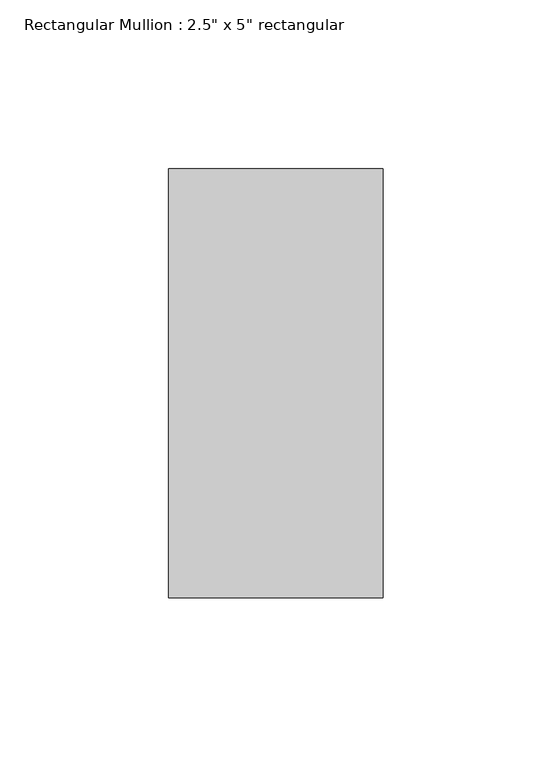
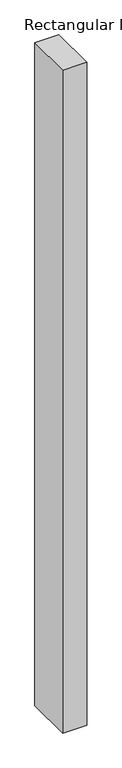
"""IFC4 building model written with IfcOpenShell, lengths in millimetres: member geometry."""

from ifc_helpers import new_model, si_unit, frame, origin, place, context, project, spatial, polyline, outline, extrude, source, transform, mapped, element, save


def member_d73967ec(model_context):
    return source(origin(), model_context, "Body", "SweptSolid", [
        extrude(outline(polyline([(31.75, 63.5), (31.75, -63.5), (-31.75, -63.5), (-31.75, 63.5), (31.75, 63.5)])), frame((0.0, 0.0, -1854.2), z_axis=(0.0, 0.0, 1.0), x_axis=(1.0, 0.0, 0.0)), (0.0, 0.0, 1.0), 1854.2),
    ])


if __name__ == "__main__":
    model = new_model("IFC4")
    model_context = context("Model", 3, world=origin())
    ifc_project = project(units=[si_unit("LENGTHUNIT", "METRE", prefix="MILLI")], contexts=[model_context])
    site = spatial("IfcSite", under=ifc_project)
    building = spatial("IfcBuilding", under=site)
    placement = place(None, origin())
    member_shape = member_d73967ec(model_context)
    element("IfcMember", 1, ObjectType="Rectangular Mullion : 2.5\" x 5\" rectangular", at=placement, inside=building, context=model_context, shape_type="MappedRepresentation", body=[
        mapped(member_shape, transform((0.0, 0.0, 0.0), x_axis=(1.0, 0.0, 0.0), y_axis=(0.0, 1.0, 0.0), z_axis=(0.0, 0.0, 1.0))),
    ])
    save(model, "model.ifc")

# Revit data of these elements
# Type "Rectangular Mullion : 2.5\" x 5\" rectangular"
#   built-in parameter 1007304 = 0.416667 (stored number, unit not read)
#   built-in parameter 1007301 = 0.104167 (stored number, unit not read)
#   built-in parameter 1007300 = 0.104167 (stored number, unit not read)
